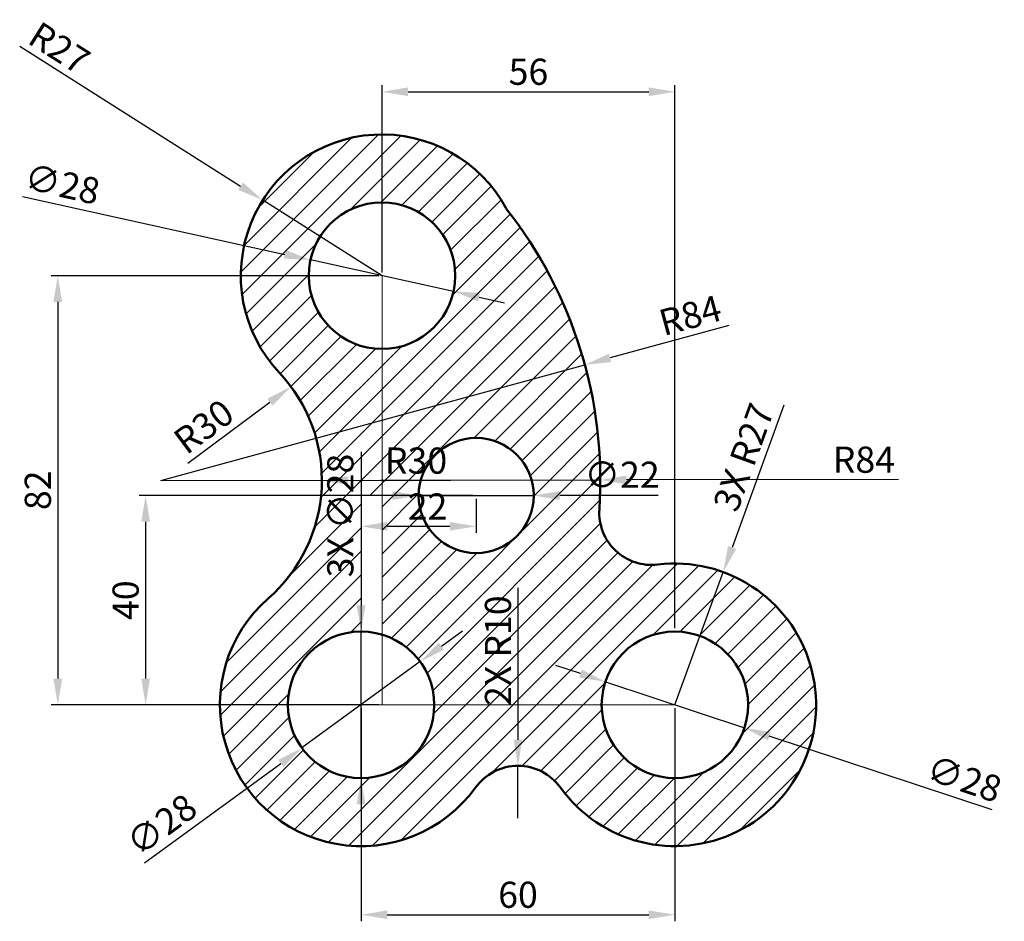
# Model space of a CAD drawing. Units: millimetres. Extents: x 877 to 1066, y 1155 to 1327.
import ezdxf

# ---------------------------------------------------------------- set-up
doc = ezdxf.new("R2010")
doc.units = ezdxf.units.MM
for name, color, linetype, lineweight in [('M-CONS', 8, 'Continuous', 18), ('M-DIMS', 2, 'Continuous', 25), ('M-HATC', 252, 'Continuous', 18), ('M-OUTL', 7, 'Continuous', 50)]:
    doc.layers.add(name, color=color, linetype=linetype, lineweight=lineweight)
doc.styles.get("Standard").update_dxf_attribs({"font": 'arial.ttf'})
doc.dimstyles.new('ISO-25', dxfattribs={"dimtxt": 5, "dimasz": 5, "dimexe": 1.25, "dimexo": 0.625, "dimtad": 1, "dimtxsty": 'Standard', "dimcen": 5, "dimadec": 0, "dimazin": 0, "dimtfac": 1, "dimtmove": 0, "dimatfit": 3, "dimfxl": 1, "dimarcsym": 0})

# ---------------------------------------------------------------- blocks, each defined once
blk = doc.blocks.new('*D1')
at = {"layer": 'Defpoints', "color": 0, "transparency": 16777216}
for p in [(954.01, 1204.48), (931.39, 1187.98)]:
    blk.add_point(p, dxfattribs=at)
at = {"layer": 'M-DIMS', "color": 0, "lineweight": -2, "transparency": 16777216}
for p, q in [((958.05, 1207.42), (962.09, 1210.37)), ((954.01, 1204.48), (931.39, 1187.98)), ((901.28, 1166.02), (927.35, 1185.03))]:
    blk.add_line(p, q, dxfattribs=at)
at = {"layer": 'M-DIMS', "color": 0, "transparency": 16777216}
for points in [[(957.56, 1208.1), (958.54, 1206.75), (954.01, 1204.48)], [(926.86, 1185.71), (927.84, 1184.36), (931.39, 1187.98)]]:
    blk.add_solid(points, dxfattribs=at)
at = {"layer": 'M-DIMS', "color": 0, "transparency": 16777216, "insert": (904.92, 1172.79), "char_height": 5, "attachment_point": 5, "rotation": 36.1026}
blk.add_mtext('∅28', dxfattribs=at)
blk = doc.blocks.new('*D2')
at = {"layer": 'Defpoints', "color": 0, "transparency": 16777216}
for p in [(942.7, 1196.23), (1002.7, 1196.23), (1002.7, 1156.11)]:
    blk.add_point(p, dxfattribs=at)
at = {"layer": 'M-DIMS', "color": 0, "lineweight": -2, "transparency": 16777216}
for p, q in [((942.7, 1195.6), (942.7, 1154.86)), ((1002.7, 1195.6), (1002.7, 1154.86)), ((947.7, 1156.11), (997.7, 1156.11))]:
    blk.add_line(p, q, dxfattribs=at)
at = {"layer": 'M-DIMS', "color": 0, "transparency": 16777216}
for points in [[(947.7, 1156.95), (947.7, 1155.28), (942.7, 1156.11)], [(997.7, 1156.95), (997.7, 1155.28), (1002.7, 1156.11)]]:
    blk.add_solid(points, dxfattribs=at)
at = {"layer": 'M-DIMS', "color": 0, "transparency": 16777216, "insert": (972.7, 1159.29), "char_height": 5, "attachment_point": 5}
blk.add_mtext('60', dxfattribs=at)
blk = doc.blocks.new('*D3')
at = {"layer": 'Defpoints', "color": 0, "transparency": 16777216}
for p in [(942.7, 1236.23), (964.7, 1236.23), (964.7, 1230.34)]:
    blk.add_point(p, dxfattribs=at)
at = {"layer": 'M-DIMS', "color": 0, "lineweight": -2, "transparency": 16777216}
for p, q in [((942.7, 1235.6), (942.7, 1229.09)), ((964.7, 1235.6), (964.7, 1229.09)), ((947.7, 1230.34), (959.7, 1230.34))]:
    blk.add_line(p, q, dxfattribs=at)
at = {"layer": 'M-DIMS', "color": 0, "transparency": 16777216}
for points in [[(947.7, 1231.17), (947.7, 1229.51), (942.7, 1230.34)], [(959.7, 1231.17), (959.7, 1229.51), (964.7, 1230.34)]]:
    blk.add_solid(points, dxfattribs=at)
at = {"layer": 'M-DIMS', "color": 0, "transparency": 16777216, "insert": (955.41, 1233.48), "char_height": 5, "attachment_point": 5}
blk.add_mtext('22', dxfattribs=at)
blk = doc.blocks.new('*D4')
at = {"layer": 'Defpoints', "color": 0, "transparency": 16777216}
for p in [(946.7, 1278.23), (884.71, 1196.23), (946.7, 1196.23)]:
    blk.add_point(p, dxfattribs=at)
at = {"layer": 'M-DIMS', "color": 0, "lineweight": -2, "transparency": 16777216}
for p, q in [((946.07, 1278.23), (883.46, 1278.23)), ((884.71, 1273.23), (884.71, 1201.23)), ((946.07, 1196.23), (883.46, 1196.23))]:
    blk.add_line(p, q, dxfattribs=at)
at = {"layer": 'M-DIMS', "color": 0, "transparency": 16777216}
for points in [[(883.87, 1273.23), (885.54, 1273.23), (884.71, 1278.23)], [(883.87, 1201.23), (885.54, 1201.23), (884.71, 1196.23)]]:
    blk.add_solid(points, dxfattribs=at)
at = {"layer": 'M-DIMS', "color": 0, "transparency": 16777216, "insert": (881.53, 1237.23), "char_height": 5, "attachment_point": 5, "rotation": 90}
blk.add_mtext('82', dxfattribs=at)
blk = doc.blocks.new('*D5')
at = {"layer": 'Defpoints', "color": 0, "transparency": 16777216}
for p in [(964.7, 1236.23), (901.5, 1196.23), (942.7, 1196.23)]:
    blk.add_point(p, dxfattribs=at)
at = {"layer": 'M-DIMS', "color": 0, "lineweight": -2, "transparency": 16777216}
for p, q in [((964.07, 1236.23), (900.25, 1236.23)), ((901.5, 1231.23), (901.5, 1201.23)), ((942.07, 1196.23), (900.25, 1196.23))]:
    blk.add_line(p, q, dxfattribs=at)
at = {"layer": 'M-DIMS', "color": 0, "transparency": 16777216}
for points in [[(900.67, 1231.23), (902.34, 1231.23), (901.5, 1236.23)], [(900.67, 1201.23), (902.34, 1201.23), (901.5, 1196.23)]]:
    blk.add_solid(points, dxfattribs=at)
at = {"layer": 'M-DIMS', "color": 0, "transparency": 16777216, "insert": (898.33, 1216.23), "char_height": 5, "attachment_point": 5, "rotation": 90}
blk.add_mtext('40', dxfattribs=at)
blk = doc.blocks.new('*D6')
at = {"layer": 'Defpoints', "color": 0, "transparency": 16777216}
for p in [(929.29, 1257.03), (905.2, 1239.16)]:
    blk.add_point(p, dxfattribs=at)
at = {"layer": 'M-DIMS', "color": 0, "lineweight": -2, "transparency": 16777216}
blk.add_line((909.59, 1242.41), (925.28, 1254.05), dxfattribs=at)
at = {"layer": 'M-DIMS', "color": 0, "transparency": 16777216}
blk.add_solid([(924.78, 1254.72), (925.77, 1253.38), (929.29, 1257.03)], dxfattribs=at)
at = {"layer": 'M-DIMS', "color": 0, "transparency": 16777216, "insert": (912.99, 1248.89), "char_height": 5, "attachment_point": 5, "rotation": 36.5764}
blk.add_mtext('R30', dxfattribs=at)
blk = doc.blocks.new('*D7')
at = {"layer": 'Defpoints', "color": 0, "transparency": 16777216}
for p in [(985.49, 1261.21), (904.44, 1239.11)]:
    blk.add_point(p, dxfattribs=at)
at = {"layer": 'M-DIMS', "color": 0, "lineweight": -2, "transparency": 16777216}
for p, q in [((1012.99, 1268.71), (990.31, 1262.52)), ((904.44, 1239.11), (985.49, 1261.21))]:
    blk.add_line(p, q, dxfattribs=at)
at = {"layer": 'M-DIMS', "color": 0, "transparency": 16777216}
blk.add_solid([(990.09, 1263.33), (990.53, 1261.72), (985.49, 1261.21)], dxfattribs=at)
at = {"layer": 'M-DIMS', "color": 0, "transparency": 16777216, "insert": (1005.8, 1270.04), "char_height": 5, "attachment_point": 5, "rotation": 15.252}
blk.add_mtext('R84', dxfattribs=at)
blk = doc.blocks.new('*D8')
at = {"layer": 'Defpoints', "color": 0, "transparency": 16777216}
for p in [(923.89, 1292.67), (946.7, 1278.23)]:
    blk.add_point(p, dxfattribs=at)
at = {"layer": 'M-DIMS', "color": 0, "lineweight": -2, "transparency": 16777216}
for p, q in [((877.42, 1322.08), (919.66, 1295.34)), ((946.7, 1278.23), (923.89, 1292.67))]:
    blk.add_line(p, q, dxfattribs=at)
at = {"layer": 'M-DIMS', "color": 0, "transparency": 16777216}
blk.add_solid([(920.11, 1296.05), (919.22, 1294.64), (923.89, 1292.67)], dxfattribs=at)
at = {"layer": 'M-DIMS', "color": 0, "transparency": 16777216, "insert": (884.68, 1321.2), "char_height": 5, "attachment_point": 5, "rotation": 327.6671}
blk.add_mtext('R27', dxfattribs=at)
blk = doc.blocks.new('*D9')
at = {"layer": 'Defpoints', "color": 0, "transparency": 16777216}
for p in [(933.03, 1281.24), (960.37, 1275.22)]:
    blk.add_point(p, dxfattribs=at)
at = {"layer": 'M-DIMS', "color": 0, "lineweight": -2, "transparency": 16777216}
for p, q in [((877.94, 1293.37), (928.14, 1282.31)), ((960.37, 1275.22), (933.03, 1281.24)), ((965.26, 1274.14), (970.14, 1273.07))]:
    blk.add_line(p, q, dxfattribs=at)
at = {"layer": 'M-DIMS', "color": 0, "transparency": 16777216}
for points in [[(928.32, 1283.13), (927.96, 1281.5), (933.03, 1281.24)], [(965.43, 1274.96), (965.08, 1273.33), (960.37, 1275.22)]]:
    blk.add_solid(points, dxfattribs=at)
at = {"layer": 'M-DIMS', "color": 0, "transparency": 16777216, "insert": (885.42, 1295.12), "char_height": 5, "attachment_point": 5, "rotation": 347.5817}
blk.add_mtext('∅28', dxfattribs=at)
blk = doc.blocks.new('*D10')
at = {"layer": 'Defpoints', "color": 0, "transparency": 16777216}
for p in [(989.41, 1200.63), (1015.99, 1191.83)]:
    blk.add_point(p, dxfattribs=at)
at = {"layer": 'M-DIMS', "color": 0, "lineweight": -2, "transparency": 16777216}
for p, q in [((984.66, 1202.2), (979.92, 1203.77)), ((989.41, 1200.63), (1015.99, 1191.83)), ((1063.36, 1176.15), (1020.74, 1190.26))]:
    blk.add_line(p, q, dxfattribs=at)
at = {"layer": 'M-DIMS', "color": 0, "transparency": 16777216}
for points in [[(984.92, 1202.99), (984.4, 1201.41), (989.41, 1200.63)], [(1021, 1191.05), (1020.48, 1189.47), (1015.99, 1191.83)]]:
    blk.add_solid(points, dxfattribs=at)
at = {"layer": 'M-DIMS', "color": 0, "transparency": 16777216, "insert": (1057.83, 1181.48), "char_height": 5, "attachment_point": 5, "rotation": 341.685}
blk.add_mtext('∅28', dxfattribs=at)
blk = doc.blocks.new('*D11')
at = {"layer": 'Defpoints', "color": 0, "transparency": 16777216}
for p in [(1002.7, 1313.38), (946.7, 1278.23), (1002.7, 1210.23)]:
    blk.add_point(p, dxfattribs=at)
at = {"layer": 'M-DIMS', "color": 0, "lineweight": -2, "transparency": 16777216}
for p, q in [((946.7, 1278.85), (946.7, 1314.63)), ((1002.7, 1210.85), (1002.7, 1314.63)), ((951.7, 1313.38), (997.7, 1313.38))]:
    blk.add_line(p, q, dxfattribs=at)
at = {"layer": 'M-DIMS', "color": 0, "transparency": 16777216}
for points in [[(951.7, 1314.22), (951.7, 1312.55), (946.7, 1313.38)], [(997.7, 1314.22), (997.7, 1312.55), (1002.7, 1313.38)]]:
    blk.add_solid(points, dxfattribs=at)
at = {"layer": 'M-DIMS', "color": 0, "transparency": 16777216, "insert": (974.7, 1316.56), "char_height": 5, "attachment_point": 5}
blk.add_mtext('56', dxfattribs=at)
blk = doc.blocks.new('*D12')
at = {"layer": 'Defpoints', "color": 0, "transparency": 16777216}
for p in [(1011.93, 1221.6), (1002.7, 1196.23)]:
    blk.add_point(p, dxfattribs=at)
at = {"layer": 'M-DIMS', "color": 0, "lineweight": -2, "transparency": 16777216}
for p, q in [((1023.54, 1253.49), (1013.65, 1226.3)), ((1002.7, 1196.23), (1011.93, 1221.6))]:
    blk.add_line(p, q, dxfattribs=at)
at = {"layer": 'M-DIMS', "color": 0, "transparency": 16777216}
blk.add_solid([(1012.86, 1226.58), (1014.43, 1226.01), (1011.93, 1221.6)], dxfattribs=at)
at = {"layer": 'M-DIMS', "color": 0, "transparency": 16777216, "insert": (1016.46, 1243.33), "char_height": 5, "attachment_point": 5, "rotation": 69.9982}
blk.add_mtext('3X R27', dxfattribs=at)
blk = doc.blocks.new('*D13')
at = {"layer": 'Defpoints', "color": 0, "transparency": 16777216}
for p in [(942.7, 1210.23), (942.7, 1182.23)]:
    blk.add_point(p, dxfattribs=at)
at = {"layer": 'M-DIMS', "color": 0, "lineweight": -2, "transparency": 16777216}
for p, q in [((942.7, 1244.56), (942.7, 1215.23)), ((942.7, 1182.23), (942.7, 1210.23)), ((942.7, 1177.23), (942.7, 1172.23))]:
    blk.add_line(p, q, dxfattribs=at)
at = {"layer": 'M-DIMS', "color": 0, "transparency": 16777216}
for points in [[(941.87, 1215.23), (943.53, 1215.23), (942.7, 1210.23)], [(941.87, 1177.23), (943.53, 1177.23), (942.7, 1182.23)]]:
    blk.add_solid(points, dxfattribs=at)
at = {"layer": 'M-DIMS', "color": 0, "transparency": 16777216, "insert": (939.38, 1232.4), "char_height": 5, "attachment_point": 5, "rotation": 89.9982}
blk.add_mtext('3X ∅28', dxfattribs=at)
blk = doc.blocks.new('*D14')
at = {"layer": 'Defpoints', "color": 0, "transparency": 16777216}
for p in [(953.7, 1236.23), (975.7, 1236.23)]:
    blk.add_point(p, dxfattribs=at)
at = {"layer": 'M-DIMS', "color": 0, "lineweight": -2, "transparency": 16777216}
for p, q in [((948.7, 1236.23), (943.7, 1236.23)), ((953.7, 1236.23), (975.7, 1236.23)), ((999.5, 1236.23), (980.7, 1236.23))]:
    blk.add_line(p, q, dxfattribs=at)
at = {"layer": 'M-DIMS', "color": 0, "transparency": 16777216}
for points in [[(948.7, 1237.06), (948.7, 1235.4), (953.7, 1236.23)], [(980.7, 1237.06), (980.7, 1235.39), (975.7, 1236.23)]]:
    blk.add_solid(points, dxfattribs=at)
at = {"layer": 'M-DIMS', "color": 0, "transparency": 16777216, "insert": (992.6, 1239.55), "char_height": 5, "attachment_point": 5, "rotation": 359.9984}
blk.add_mtext('∅22', dxfattribs=at)
blk = doc.blocks.new('*D15')
at = {"layer": 'Defpoints', "color": 0, "transparency": 16777216}
for p in [(972.7, 1184.57), (972.7, 1174.57)]:
    blk.add_point(p, dxfattribs=at)
at = {"layer": 'M-DIMS', "color": 0, "lineweight": -2, "transparency": 16777216}
for p, q in [((972.7, 1218.58), (972.7, 1189.57)), ((972.7, 1174.57), (972.7, 1184.57))]:
    blk.add_line(p, q, dxfattribs=at)
at = {"layer": 'M-DIMS', "color": 0, "transparency": 16777216}
blk.add_solid([(971.87, 1189.57), (973.53, 1189.57), (972.7, 1184.57)], dxfattribs=at)
at = {"layer": 'M-DIMS', "color": 0, "transparency": 16777216, "insert": (969.52, 1206.58), "char_height": 5, "attachment_point": 5, "rotation": 89.9975}
blk.add_mtext('2X R10', dxfattribs=at)
blk = doc.blocks.new('*D16')
at = {"layer": 'Defpoints', "color": 0, "transparency": 16777216}
for p in [(905.2, 1239.16), (935.2, 1239.1)]:
    blk.add_point(p, dxfattribs=at)
at = {"layer": 'M-DIMS', "color": 0, "lineweight": -2, "transparency": 16777216}
for p, q in [((905.2, 1239.16), (935.2, 1239.1)), ((959.79, 1239.05), (940.2, 1239.09))]:
    blk.add_line(p, q, dxfattribs=at)
at = {"layer": 'M-DIMS', "color": 0, "transparency": 16777216}
blk.add_solid([(940.2, 1239.92), (940.2, 1238.26), (935.2, 1239.1)], dxfattribs=at)
at = {"layer": 'M-DIMS', "color": 0, "transparency": 16777216, "insert": (953.2, 1242.25), "char_height": 5, "attachment_point": 5, "rotation": 359.8945}
blk.add_mtext('R30', dxfattribs=at)
blk = doc.blocks.new('*D17')
at = {"layer": 'Defpoints', "color": 0, "transparency": 16777216}
for p in [(904.44, 1239.11), (988.44, 1239.2)]:
    blk.add_point(p, dxfattribs=at)
at = {"layer": 'M-DIMS', "color": 0, "lineweight": -2, "transparency": 16777216}
for p, q in [((904.44, 1239.11), (988.44, 1239.2)), ((1045.43, 1239.26), (993.44, 1239.21))]:
    blk.add_line(p, q, dxfattribs=at)
at = {"layer": 'M-DIMS', "color": 0, "transparency": 16777216}
blk.add_solid([(993.44, 1240.04), (993.44, 1238.37), (988.44, 1239.2)], dxfattribs=at)
at = {"layer": 'M-DIMS', "color": 0, "transparency": 16777216, "insert": (1038.84, 1242.43), "char_height": 5, "attachment_point": 5, "rotation": 0.0624}
blk.add_mtext('R84', dxfattribs=at)

msp = doc.modelspace()

# ---------------------------------------------------------------- hatches: boundary and pattern name
at = {"layer": 'M-HATC'}
h = msp.add_hatch(dxfattribs=at)
h.set_pattern_fill('ANSI31', color=256)
h.paths.add_polyline_path([(970.464, 1291.044, 1.1396434), (927.041, 1259.72, -0.4251666), (924.936, 1216.562, 1.1207507), (964.591, 1180.425, -0.5114531), (980.808, 1180.425, 1.7513038), (999.447, 1223.032, -0.4698707), (988.264, 1233.613, 0.1850777)])
h.paths.add_polyline_path([(946.7, 1264.228), (946.7, 1236.228), (953.7, 1236.228, -1), (975.7, 1236.228, -1), (953.7, 1236.228), (946.7, 1236.228), (946.7, 1209.645, -0.3316793), (956.7, 1196.228), (988.7, 1196.228, -1), (1016.7, 1196.228, -1), (988.7, 1196.228), (956.7, 1196.228, -1), (928.7, 1196.228, -0.4142136), (942.7, 1210.228), (942.7, 1236.228), (946.7, 1236.228), (946.7, 1264.228, -0.4142136), (932.7, 1278.228, -1), (960.7, 1278.228, -0.4142136)], flags=16)
h.paths.add_polyline_path([(950.355, 1228.235), (960.625, 1228.235), (960.625, 1238.538), (950.355, 1238.538)], flags=24)

# ---------------------------------------------------------------- linework, layer by layer
at = {"layer": 'M-CONS'}
for p, q in [((946.7, 1196.228), (946.7, 1278.228)), ((942.7, 1196.228), (942.7, 1236.228)), ((942.7, 1236.228), (964.7, 1236.228)), ((942.7, 1196.228), (1002.7, 1196.228)), ((942.7, 1196.228), (946.7, 1196.228))]:
    msp.add_line(p, q, dxfattribs=at)
at = {"layer": 'M-OUTL'}
for centre, radius in [((946.7, 1278.228), 14), ((964.7, 1236.228), 11), ((942.7, 1196.228), 14), ((1002.7, 1196.228), 14)]:
    msp.add_circle(centre, radius, dxfattribs=at)
for centre, radius, start, end in [((946.7, 1278.228), 27, 28.33805, 223.27446), ((904.444, 1239.108), 84, 356.24895, 38.19104), ((905.199, 1239.155), 30, 311.14014, 43.27446), ((998.242, 1232.959), 10, 176.24895, 276.91876), ((1002.7, 1196.228), 27, 215.82477, 96.91876), ((942.7, 1196.228), 27, 131.14014, 324.17523), ((972.7, 1174.572), 10, 35.82477, 144.17523)]:
    msp.add_arc(centre, radius, start, end, dxfattribs=at)

# ---------------------------------------------------------------- dimensions: what is measured, and where the dimension line sits
at = {"layer": 'M-DIMS'}
for center, mpoint, override, picture, middle in [((946.7, 1278.228), (923.886, 1292.669), {"dimclrd": 0, "dimclre": 0, "dimclrt": 0}, '*D8', (882.999, 1318.55)), ((904.444, 1239.108), (985.485, 1261.206), {"dimclrd": 0, "dimclre": 0, "dimclrt": 0}, '*D7', (1006.636, 1266.973)), ((905.199, 1239.155), (929.291, 1257.032), {"dimclrd": 0, "dimclre": 0, "dimclrt": 0}, '*D6', (914.88, 1246.339)), ((904.444, 1239.108), (988.444, 1239.2), {"dimdec": 0, "dimlfac": 1, "dimrnd": 0, "dimzin": 0, "dimdsep": 46, "dimlunit": 2}, '*D17', (1038.844, 1239.255)), ((905.199, 1239.155), (935.199, 1239.1), {"dimdec": 0, "dimlfac": 1, "dimrnd": 0, "dimzin": 0, "dimdsep": 46, "dimlunit": 2}, '*D16', (953.199, 1239.067))]:
    dim = msp.add_radius_dim(center=center, mpoint=mpoint, dimstyle='ISO-25', override=override, dxfattribs=at)
    dim.commit()
    dim.dimension.update_dxf_attribs({"geometry": picture, "text_midpoint": middle, "dimtype": 164})
for base, p1, p2, picture, middle in [((1002.7, 1313.382), (946.7, 1278.228), (1002.7, 1210.228), '*D11', (974.7, 1316.56)), ((1002.7, 1156.112), (942.7, 1196.228), (1002.7, 1196.228), '*D2', (972.7, 1159.29))]:
    dim = msp.add_linear_dim(base=base, p1=p1, p2=p2, dimstyle='ISO-25', override={"dimclrd": 0, "dimclre": 0, "dimclrt": 0}, dxfattribs=at)
    dim.commit()
    dim.dimension.update_dxf_attribs({"geometry": picture, "text_midpoint": middle})
for p1, p2, override, picture, middle in [((960.372, 1275.218), (933.027, 1281.239), {"dimclrd": 0, "dimclre": 0, "dimclrt": 0}, '*D9', (884.708, 1291.879)), ((953.7, 1236.229), (975.7, 1236.228), {"dimdec": 0, "dimlfac": 1, "dimrnd": 0, "dimzin": 0, "dimdsep": 46, "dimlunit": 2}, '*D14', (992.6, 1236.228)), ((954.011, 1204.478), (931.388, 1187.979), {"dimclrd": 0, "dimclre": 0, "dimclrt": 0}, '*D1', (906.878, 1170.105)), ((989.409, 1200.628), (1015.99, 1191.829), {"dimclrd": 0, "dimclre": 0, "dimclrt": 0}, '*D10', (1056.784, 1178.326))]:
    dim = msp.add_diameter_dim_2p(p1=p1, p2=p2, dimstyle='ISO-25', override=override, dxfattribs=at)
    dim.commit()
    dim.dimension.update_dxf_attribs({"geometry": picture, "text_midpoint": middle, "dimtype": 163})
for base, p1, p2, picture, middle in [((884.708, 1196.228), (946.7, 1278.228), (946.7, 1196.228), '*D4', (881.53, 1237.228)), ((901.504, 1196.228), (964.7, 1236.228), (942.7, 1196.228), '*D5', (898.326, 1216.228))]:
    dim = msp.add_linear_dim(base=base, p1=p1, p2=p2, angle=90, dimstyle='ISO-25', override={"dimclrd": 0, "dimclre": 0, "dimclrt": 0}, dxfattribs=at)
    dim.commit()
    dim.dimension.update_dxf_attribs({"geometry": picture, "text_midpoint": middle})
for center, mpoint, text, picture, middle in [((1002.7, 1196.228), (1011.935, 1221.6), '3X <>', '*D12', (1016.462, 1243.331)), ((972.7, 1174.572), (972.7, 1184.572), '2X <>', '*D15', (969.523, 1206.577))]:
    dim = msp.add_radius_dim(center=center, mpoint=mpoint, text=text, dimstyle='ISO-25', override={"dimdec": 0, "dimlfac": 1, "dimrnd": 0, "dimzin": 0, "dimdsep": 46, "dimlunit": 2}, dxfattribs=at)
    dim.commit()
    dim.dimension.update_dxf_attribs({"geometry": picture, "text_midpoint": middle})
dim = msp.add_diameter_dim_2p(p1=(942.699, 1182.228), p2=(942.7, 1210.228), text='3X <>', dimstyle='ISO-25', override={"dimdec": 0, "dimlfac": 1, "dimrnd": 0, "dimzin": 0, "dimdsep": 46, "dimlunit": 2}, dxfattribs=at)
dim.commit()
dim.dimension.update_dxf_attribs({"geometry": '*D13', "text_midpoint": (942.701, 1232.397), "dimtype": 163})
dim = msp.add_linear_dim(base=(964.7, 1230.34), p1=(942.7, 1236.228), p2=(964.7, 1236.228), dimstyle='ISO-25', override={"dimclrd": 0, "dimclre": 0, "dimclrt": 0}, dxfattribs=at)
dim.commit()
dim.dimension.update_dxf_attribs({"geometry": '*D3', "text_midpoint": (955.408, 1230.34), "dimtype": 160})

doc.saveas('drawing.dxf')
